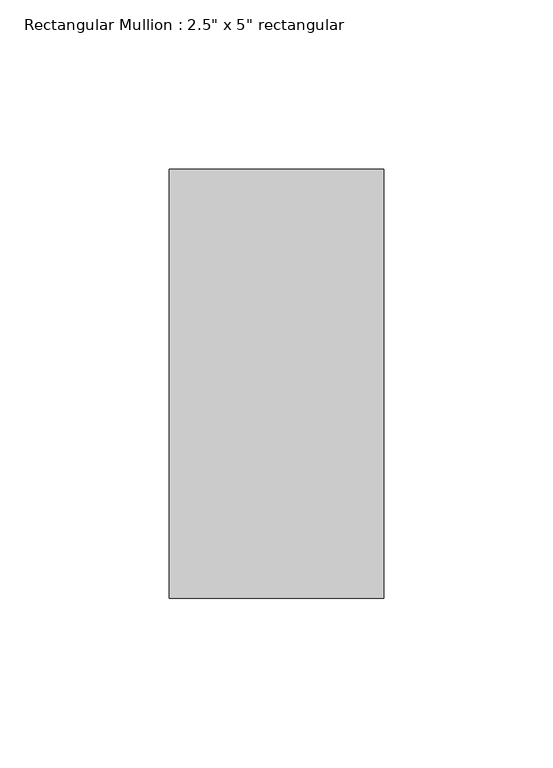
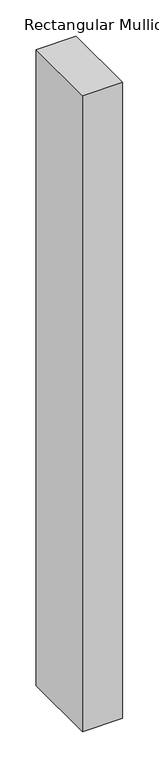
"""IFC4 building model written with IfcOpenShell, lengths in millimetres: member geometry."""

from ifc_helpers import new_model, si_unit, frame, origin, place, context, project, spatial, polyline, outline, extrude, source, transform, mapped, element, save


def member_c4de40ee(model_context):
    return source(origin(), model_context, "Body", "SweptSolid", [
        extrude(outline(polyline([(0.0, 63.5), (0.0, -63.5), (-63.5, -63.5), (-63.5, 63.5), (0.0, 63.5)])), frame((0.0, 0.0, -1066.8), z_axis=(0.0, 0.0, 1.0), x_axis=(1.0, 0.0, 0.0)), (0.0, 0.0, 1.0), 1066.8),
    ])


if __name__ == "__main__":
    model = new_model("IFC4")
    model_context = context("Model", 3, world=origin())
    ifc_project = project(units=[si_unit("LENGTHUNIT", "METRE", prefix="MILLI")], contexts=[model_context])
    site = spatial("IfcSite", under=ifc_project)
    building = spatial("IfcBuilding", under=site)
    placement = place(None, origin())
    member_shape = member_c4de40ee(model_context)
    element("IfcMember", 1, ObjectType="Rectangular Mullion : 2.5\" x 5\" rectangular", at=placement, inside=building, context=model_context, shape_type="MappedRepresentation", body=[
        mapped(member_shape, transform((0.0, 0.0, 0.0), x_axis=(1.0, 0.0, 0.0), y_axis=(0.0, 1.0, 0.0), z_axis=(0.0, 0.0, 1.0))),
    ])
    save(model, "model.ifc")

# Revit data of these elements
# Type "Rectangular Mullion : 2.5\" x 5\" rectangular"
#   built-in parameter 1007304 = 0.416667 (stored number, unit not read)
#   built-in parameter 1007301 = 0.104167 (stored number, unit not read)
#   built-in parameter 1007300 = 0.104167 (stored number, unit not read)
# Element 1 (IfcMember, "Rectangular Mullion : 2.5\" x 5\" rectangular")
#   Materials on its faces: "Aluminum"
# Materials
#   "Aluminum": class "Metal", colour RGB 247 247 247, transparency 0, Description = "Aluminum 6061", Cost = 0
